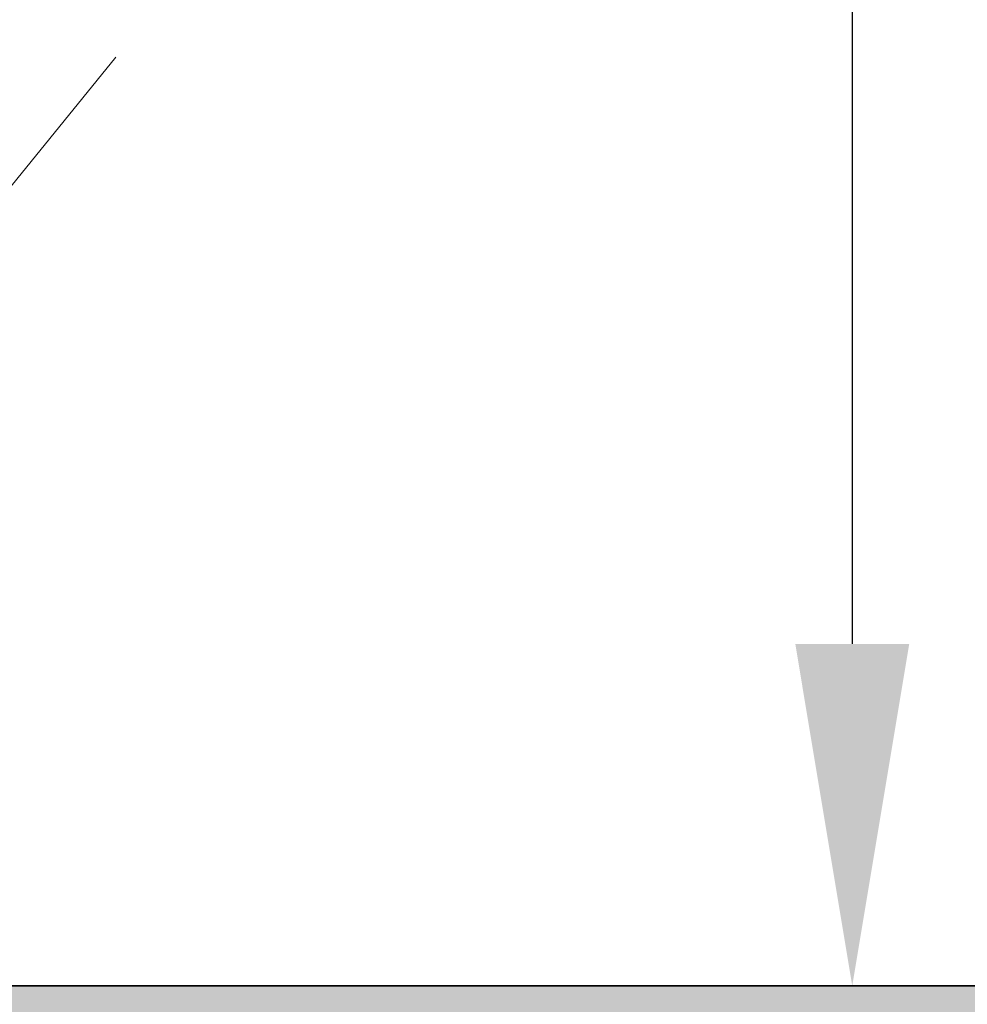
# Model space of a CAD drawing. Units: inches. Extents: x 2083 to 3317, y 1141 to 2115.
# Tile 79 of 256: x 2259 to 2292, y 1477 to 1512. Entities that reach past the tile are written whole.
import ezdxf

# ---------------------------------------------------------------- set-up
doc = ezdxf.new("R2010")
doc.units = ezdxf.units.IN
doc.linetypes.add('ACAD_ISO02W100', pattern=[15, 12, -3])
for name, color, linetype, lineweight in [('A-ANNO-DIMS', 2, 'Continuous', 18), ('A-FLOR-OPEN', 8, 'ACAD_ISO02W100', 13), ('A-WALL', 7, 'Continuous', 35)]:
    doc.layers.add(name, color=color, linetype=linetype, lineweight=lineweight)
doc.layers.add('A-WALL-PATT', color=251, linetype='Continuous', lineweight=13, true_color=0x636466)
doc.styles.get("Standard").update_dxf_attribs({"font": 'arial.ttf'})
doc.dimstyles.new('ISO-25', dxfattribs={"dimtxt": 12, "dimasz": 12, "dimexe": 1.25, "dimexo": 0.625, "dimtad": 1, "dimlunit": 3, "dimtxsty": 'Standard', "dimcen": 2.5, "dimadec": 0, "dimazin": 0, "dimtfac": 1, "dimtmove": 0, "dimatfit": 3, "dimfxl": 1, "dimarcsym": 0})

# ---------------------------------------------------------------- blocks, each defined once
blk = doc.blocks.new('*D30')
at = {"layer": 'A-ANNO-DIMS', "color": 0, "lineweight": -2, "transparency": 16777216}
for p, q in [((2240.018, 1445.274), (2240.018, 1448.046)), ((2254.329, 1445.274), (2254.329, 1448.046)), ((2228.018, 1446.796), (2216.018, 1446.796)), ((2240.018, 1446.796), (2254.329, 1446.796)), ((2266.329, 1446.796), (2413.765, 1446.796))]:
    blk.add_line(p, q, dxfattribs=at)
at = {"layer": 'A-ANNO-DIMS', "color": 0, "transparency": 16777216}
for points in [[(2228.018, 1448.796), (2228.018, 1444.796), (2240.018, 1446.796)], [(2266.329, 1448.796), (2266.329, 1444.796), (2254.329, 1446.796)]]:
    blk.add_solid(points, dxfattribs=at)
at = {"layer": 'Defpoints', "color": 0, "transparency": 16777216}
for p in [(2254.329, 1446.796), (2240.018, 1444.649), (2254.329, 1444.649)]:
    blk.add_point(p, dxfattribs=at)
at = {"layer": 'A-ANNO-DIMS', "color": 0, "transparency": 16777216, "insert": (2346.047, 1453.625), "char_height": 12, "attachment_point": 5}
blk.add_mtext('WC 1\'-2 1/2" TYP.', dxfattribs=at)
blk = doc.blocks.new('*D45')
at = {"layer": 'A-ANNO-DIMS', "color": 0, "lineweight": -2, "transparency": 16777216}
for p, q in [((2235.96, 1478.386), (2235.96, 1531.361)), ((2418.96, 1478.386), (2418.96, 1531.361)), ((2247.96, 1530.111), (2406.96, 1530.111))]:
    blk.add_line(p, q, dxfattribs=at)
at = {"layer": 'A-ANNO-DIMS', "color": 0, "transparency": 16777216}
for points in [[(2247.96, 1532.111), (2247.96, 1528.111), (2235.96, 1530.111)], [(2406.96, 1532.111), (2406.96, 1528.111), (2418.96, 1530.111)]]:
    blk.add_solid(points, dxfattribs=at)
at = {"layer": 'Defpoints', "color": 0, "transparency": 16777216}
for p in [(2418.96, 1530.111), (2235.96, 1477.761), (2418.96, 1477.761)]:
    blk.add_point(p, dxfattribs=at)
at = {"layer": 'A-ANNO-DIMS', "color": 0, "transparency": 16777216, "insert": (2327.46, 1536.867), "char_height": 12, "attachment_point": 5}
blk.add_mtext('15\'-3"', dxfattribs=at)
blk = doc.blocks.new('*D62')
at = {"layer": 'A-ANNO-DIMS', "color": 0, "lineweight": -2, "transparency": 16777216}
for p, q in [((2235.96, 1469.386), (2235.96, 1522.361)), ((2379.96, 1469.386), (2379.96, 1522.361)), ((2247.96, 1521.111), (2367.96, 1521.111))]:
    blk.add_line(p, q, dxfattribs=at)
at = {"layer": 'A-ANNO-DIMS', "color": 0, "transparency": 16777216}
for points in [[(2247.96, 1523.111), (2247.96, 1519.111), (2235.96, 1521.111)], [(2367.96, 1523.111), (2367.96, 1519.111), (2379.96, 1521.111)]]:
    blk.add_solid(points, dxfattribs=at)
at = {"layer": 'Defpoints', "color": 0, "transparency": 16777216}
for p in [(2379.96, 1521.111), (2235.96, 1468.761), (2379.96, 1468.761)]:
    blk.add_point(p, dxfattribs=at)
at = {"layer": 'A-ANNO-DIMS', "color": 0, "transparency": 16777216, "insert": (2307.96, 1527.863), "char_height": 12, "attachment_point": 5}
blk.add_mtext('12\'-0"', dxfattribs=at)
blk = doc.blocks.new('*D64')
at = {"layer": 'A-ANNO-DIMS', "color": 0, "lineweight": -2, "transparency": 16777216}
for p, q in [((2236.585, 1702.761), (2289.56, 1702.761)), ((2288.31, 1690.761), (2288.31, 1489.761)), ((2236.585, 1477.761), (2289.56, 1477.761))]:
    blk.add_line(p, q, dxfattribs=at)
at = {"layer": 'A-ANNO-DIMS', "color": 0, "transparency": 16777216}
for points in [[(2286.31, 1690.761), (2290.31, 1690.761), (2288.31, 1702.761)], [(2286.31, 1489.761), (2290.31, 1489.761), (2288.31, 1477.761)]]:
    blk.add_solid(points, dxfattribs=at)
at = {"layer": 'Defpoints', "color": 0, "transparency": 16777216}
for p in [(2235.96, 1702.761), (2235.96, 1477.761), (2288.31, 1477.761)]:
    blk.add_point(p, dxfattribs=at)
at = {"layer": 'A-ANNO-DIMS', "color": 0, "transparency": 16777216, "insert": (2281.558, 1590.261), "char_height": 12, "attachment_point": 5, "rotation": 90}
blk.add_mtext('18\'-9"', dxfattribs=at)

msp = doc.modelspace()

# ---------------------------------------------------------------- hatches: boundary and pattern name
at = {"layer": 'A-WALL-PATT'}
h = msp.add_hatch(color=256, dxfattribs=at)
h.dxf.hatch_style = 1
h.paths.add_polyline_path([(3126.96, 2020.761), (2748.96, 2020.761), (2604.96, 2020.761), (2226.96, 2020.761), (2226.96, 1702.761), (2466.96, 1702.761), (2466.96, 1582.761), (2418.96, 1582.761), (2418.96, 1477.761), (2226.96, 1477.761), (2226.96, 1263.261), (2544.96, 1263.261), (2544.96, 1411.761), (2604.96, 1411.761), (2685.96, 1411.761), (2685.96, 1420.761), (2604.96, 1420.761), (2604.96, 1573.761), (2604.96, 1702.761), (2604.96, 2011.761), (2748.96, 2011.761), (2748.96, 1702.761), (2862.96, 1702.761), (2862.96, 1621.761), (2871.96, 1621.761), (2871.96, 1702.761), (2883.96, 1702.761), (2883.96, 1706.939, -0.026459), (2883.96, 1711.761), (2757.96, 1711.761), (2757.96, 1807.761), (2787.96, 1807.761), (2787.96, 1812.261), (2757.96, 1812.261), (2757.96, 2011.761), (2877.96, 2011.761), (2877.96, 1812.261), (2847.96, 1812.261), (2847.96, 1807.761), (2889.836, 1807.761), (2889.836, 1812.261), (2882.46, 1812.261), (2882.46, 2011.761), (3117.96, 2011.761), (3117.96, 1812.261), (2937.836, 1812.261), (2937.836, 1807.761), (2995.71, 1807.761), (2995.71, 1796.118), (3000.21, 1796.118), (3000.21, 1807.761), (3117.96, 1807.761), (3117.96, 1711.761), (3000.21, 1711.761), (3000.21, 1760.118), (2998.573, 1760.118, -0.020711), (2995.71, 1760.118), (2995.71, 1711.761), (2931.96, 1711.761), (2931.96, 1702.761), (3126.96, 1702.761)])
h.paths.add_polyline_path([(2471.46, 2011.761), (2471.46, 1810.011), (2462.717, 1810.011), (2462.717, 1805.511), (2505.96, 1805.511), (2505.96, 1810.011), (2475.96, 1810.011), (2475.96, 2011.761), (2595.96, 2011.761), (2595.96, 1810.011), (2565.96, 1810.011), (2565.96, 1805.511), (2595.96, 1805.511), (2595.96, 1711.761), (2235.96, 1711.761), (2235.96, 1805.511), (2353.71, 1805.511), (2353.71, 1796.054), (2358.21, 1796.054), (2358.21, 1805.511), (2414.717, 1805.511), (2414.717, 1810.011), (2235.96, 1810.011), (2235.96, 2011.761)], flags=16)
h.paths.add_polyline_path([(2270.205, 1994.61), (2270.205, 1970.61), (2246.205, 1970.61), (2246.205, 1994.61)], flags=0)
edge = h.paths.add_edge_path(flags=0)
edge.add_ellipse((2332.027, 1899.798), major_axis=(-3.043, 3.043), ratio=0.168252, start_angle=-161.3322, end_angle=-156.3071, ccw=False)
edge.add_ellipse((2333.082, 1898.744), major_axis=(-1.055, 1.055), ratio=0.453532, start_angle=-123.371, end_angle=-94.1591)
edge = h.paths.add_edge_path(flags=0)
edge.add_ellipse((2332.027, 1968.876), major_axis=(3.043, 3.043), ratio=0.168252, start_angle=18.6678, end_angle=23.6929)
edge.add_spline(control_points=[(2332.926, 1970.691), (2332.227, 1970.336), (2330.894, 1969.659), (2328.413, 1970.932), (2327.204, 1967.749), (2324.71, 1969.956), (2322.533, 1967.012), (2320.013, 1971.296), (2317.68, 1968.158), (2316.041, 1967.102), (2315.427, 1966.81)], knot_values=[0, 0, 0, 0, 2.267059, 4.324559, 6.685584, 8.878641, 11.121502, 14.300359, 17.755284, 19.732645, 19.732645, 19.732645, 19.732645], degree=3, periodic=0)
edge.add_ellipse((2332.027, 1968.876), major_axis=(3.043, 3.043), ratio=0.168252, start_angle=18.6678, end_angle=23.6929, ccw=False)
edge.add_ellipse((2333.082, 1969.931), major_axis=(1.055, 1.055), ratio=0.453532, start_angle=56.629, end_angle=85.8409, ccw=False)
edge = h.paths.add_edge_path(flags=0)
edge.add_spline(control_points=[(2296.428, 1967.988), (2293.628, 1965.336), (2287.704, 1959.727), (2299.744, 1949.996), (2294.533, 1935.669), (2290.573, 1920.604), (2293.394, 1909.974), (2296.185, 1904.967)], knot_values=[0.099185, 0.099185, 0.099185, 0.099185, 0.345301, 0.619822, 0.982653, 1.386093, 1.810555, 1.810555, 1.810555, 1.810555], degree=3, periodic=0)
edge.add_spline(control_points=[(2296.185, 1904.967), (2297.384, 1902.619), (2298.001, 1901.949), (2298.553, 1901.468)], knot_values=[0.006246, 0.006246, 0.006246, 0.006246, 0.055476, 0.055476, 0.055476, 0.055476], degree=3, periodic=0)
edge.add_spline(control_points=[(2298.553, 1901.468), (2297.259, 1900.923), (2295.225, 1900.232), (2293.06, 1900.614), (2292.101, 1900.788), (2292.09, 1900.791)], knot_values=[0.312835, 0.312835, 0.312835, 0.312835, 0.40178, 0.474987, 0.475903, 0.475903, 0.475903, 0.475903], degree=3, periodic=0)
edge.add_arc((2292.794, 1904.664), 3.937, 215.4209, 259.6982, ccw=False)
edge.add_spline(control_points=[(2289.585, 1902.382), (2289.477, 1902.535), (2289.368, 1902.688), (2289.261, 1902.841)], knot_values=[0.102872, 0.102872, 0.102872, 0.102872, 0.116896, 0.116896, 0.116896, 0.116896], degree=3, periodic=0)
edge.add_spline(control_points=[(2289.261, 1902.841), (2288.687, 1902.55), (2287.64, 1902.02), (2285.881, 1901.874), (2283.853, 1901.504), (2281.72, 1899.711), (2278.467, 1899.493), (2276.157, 1901.883), (2272.259, 1899.804), (2267.778, 1901.843), (2262.244, 1900.184), (2257.415, 1901.782), (2254.318, 1900.726), (2253.178, 1900.337)], knot_values=[0, 0, 0, 0, 1.907977, 3.477176, 5.261074, 7.972851, 11.680248, 13.717921, 16.939592, 22.789562, 27.502503, 33.595215, 37.145618, 37.145618, 37.145618, 37.145618], degree=3, periodic=0)
edge.add_line((2253.178, 1900.337), (2250.244, 1902.841))
edge.add_line((2250.244, 1902.841), (2250.244, 1965.833))
edge.add_line((2250.244, 1965.833), (2253.178, 1968.337))
edge.add_spline(control_points=[(2253.178, 1968.337), (2254.318, 1967.948), (2257.415, 1966.892), (2262.244, 1968.49), (2267.778, 1966.831), (2271.527, 1968.537), (2273.876, 1967.828), (2274.207, 1967.728)], knot_values=[0, 0, 0, 0, 0.09018, 0.244935, 0.364644, 0.513233, 0.537855, 0.537855, 0.537855, 0.537855], degree=3, periodic=0)
edge.add_arc((2274.353, 1963.793), 3.937, 72.0511, 92.1279, ccw=False)
edge.add_arc((2281.297, 1985.23), 18.596, 252.0511, 288.5657)
edge.add_arc((2292.317, 1956.029), 12.646, 71.0268, 113.7782, ccw=False)
edge = h.paths.add_edge_path(flags=0)
edge.add_spline(control_points=[(2274.899, 1951.856), (2275.066, 1951.617), (2275.233, 1951.377), (2275.398, 1951.136)], knot_values=[1.409916, 1.409916, 1.409916, 1.409916, 1.43159, 1.43159, 1.43159, 1.43159], degree=3, periodic=0)
edge.add_spline(control_points=[(2275.398, 1951.136), (2275.792, 1950.562), (2276.179, 1949.984), (2276.546, 1949.397)], knot_values=[1.358238, 1.358238, 1.358238, 1.358238, 1.409916, 1.409916, 1.409916, 1.409916], degree=3, periodic=0)
edge.add_line((2276.546, 1949.397), (2277.437, 1947.862))
edge.add_spline(control_points=[(2277.437, 1947.862), (2276.304, 1945.673), (2274.64, 1942.427), (2274.632, 1938.094), (2272.799, 1930.852), (2274.356, 1943.897), (2275.948, 1947.923), (2276.546, 1949.397)], knot_values=[0.005632, 0.005632, 0.005632, 0.005632, 0.186014, 0.266002, 0.357087, 0.59639, 0.739732, 0.739732, 0.739732, 0.739732], degree=3, periodic=0)
edge.add_spline(control_points=[(2276.546, 1949.397), (2276.179, 1949.984), (2275.792, 1950.562), (2275.398, 1951.136)], knot_values=[1.358238, 1.358238, 1.358238, 1.358238, 1.409916, 1.409916, 1.409916, 1.409916], degree=3, periodic=0)
edge.add_spline(control_points=[(2275.398, 1951.136), (2274.943, 1950.08), (2274.208, 1948.025), (2273.935, 1944.851), (2272.469, 1937.627), (2273.466, 1945.696), (2274.701, 1951.059), (2274.899, 1951.856)], knot_values=[0.104364, 0.104364, 0.104364, 0.104364, 0.189636, 0.269624, 0.36071, 0.600013, 0.644622, 0.644622, 0.644622, 0.644622], degree=3, periodic=0)
h.paths.add_polyline_path([(2269.168, 1963.128, -0.357527), (2268.171, 1960.976, -0.092561), (2268.171, 1939.436, -0.357527), (2269.168, 1937.285, -0.357527), (2267.016, 1938.282, -0.164785), (2254.686, 1938.282, -0.357527), (2252.534, 1937.285, -0.357527), (2253.531, 1939.436, -0.092561), (2253.531, 1960.976, -0.357527), (2252.534, 1963.128, -0.357527), (2254.686, 1962.131, -0.164785), (2267.016, 1962.131, -0.357527)], flags=0)
h.paths.add_polyline_path([(2248.874, 1967.802), (2248.874, 1957.028), (2249.458, 1957.028), (2249.458, 1911.647), (2248.874, 1911.647), (2248.874, 1900.873), (2246.512, 1900.873, 0.197327), (2244.15, 1902.457), (2244.15, 1966.218, 0.197327), (2246.512, 1967.802)], flags=0)
h.paths.add_polyline_path([(2269.168, 1931.389, -0.357527), (2268.171, 1929.238, -0.092561), (2268.171, 1907.698, -0.357527), (2269.168, 1905.547, -0.357527), (2267.016, 1906.544, -0.164785), (2254.686, 1906.544, -0.357527), (2252.534, 1905.547, -0.357527), (2253.531, 1907.698, -0.092561), (2253.531, 1929.238, -0.357527), (2252.534, 1931.389, -0.357527), (2254.686, 1930.392, -0.164785), (2267.016, 1930.392, -0.357527)], flags=0)
edge = h.paths.add_edge_path(flags=0)
edge.add_spline(control_points=[(2276.197, 1906.724), (2276.168, 1909.029), (2276.114, 1913.372), (2270.598, 1924.925), (2273.905, 1919.013), (2275.922, 1916.262), (2275.475, 1912.402), (2277.258, 1910.381), (2276.696, 1908.225), (2276.646, 1906.813), (2276.618, 1906.008)], knot_values=[0, 0, 0, 0, 8.61026, 16.221274, 18.843057, 23.804898, 27.440828, 29.356102, 31.203478, 33.650687, 33.650687, 33.650687, 33.650687], degree=3, periodic=0)
edge.add_spline(control_points=[(2276.618, 1906.008), (2276.623, 1905.624), (2276.498, 1904.629), (2275.442, 1903.855), (2274.937, 1903.08), (2274.859, 1902.841)], knot_values=[0.156488, 0.156488, 0.156488, 0.156488, 0.184398, 0.231376, 0.250598, 0.250598, 0.250598, 0.250598], degree=3, periodic=0)
edge.add_line((2274.859, 1902.841), (2276.506, 1902.841))
edge.add_spline(control_points=[(2276.506, 1902.841), (2276.788, 1903.085), (2277.665, 1904.125), (2278.25, 1904.341), (2277.654, 1908.527), (2278.156, 1906.228), (2278.1, 1905.286), (2278.847, 1904.069), (2277.857, 1903.415), (2277.874, 1902.991), (2277.904, 1902.841)], knot_values=[0.059574, 0.059574, 0.059574, 0.059574, 0.080753, 0.103741, 0.16972, 0.176036, 0.207137, 0.240474, 0.262341, 0.27366, 0.27366, 0.27366, 0.27366], degree=3, periodic=0)
edge.add_line((2277.904, 1902.841), (2280.03, 1902.841))
edge.add_spline(control_points=[(2280.03, 1902.841), (2279.888, 1903.088), (2279.499, 1903.982), (2280.152, 1905.939), (2278.104, 1909.658), (2279.762, 1907.185), (2280.328, 1904.875), (2280.485, 1903.49), (2281.463, 1903.249), (2281.758, 1902.936), (2281.834, 1902.841)], knot_values=[0.013856, 0.013856, 0.013856, 0.013856, 0.034874, 0.088867, 0.107879, 0.126738, 0.158714, 0.193757, 0.217487, 0.226722, 0.226722, 0.226722, 0.226722], degree=3, periodic=0)
edge.add_spline(control_points=[(2281.834, 1902.841), (2281.788, 1902.827), (2281.647, 1902.783), (2281.396, 1902.859), (2281.088, 1902.985), (2280.721, 1903.061), (2280.333, 1903.026), (2280.125, 1902.899), (2280.03, 1902.841)], knot_values=[0, 0, 0, 0, 0.14413, 0.435517, 0.749276, 1.153046, 1.548371, 1.878348, 1.878348, 1.878348, 1.878348], degree=3, periodic=0)
edge.add_line((2280.03, 1902.841), (2277.904, 1902.841))
edge.add_spline(control_points=[(2277.904, 1902.841), (2277.893, 1902.796), (2277.865, 1902.68), (2277.607, 1902.687), (2277.274, 1902.801), (2276.838, 1902.62), (2276.584, 1902.789), (2276.506, 1902.841)], knot_values=[0, 0, 0, 0, 0.127189, 0.326199, 0.628009, 1.24357, 1.515331, 1.515331, 1.515331, 1.515331], degree=3, periodic=0)
edge.add_line((2276.506, 1902.841), (2274.859, 1902.841))
edge.add_spline(control_points=[(2274.859, 1902.841), (2274.814, 1902.899), (2274.725, 1903.013), (2274.493, 1903.119), (2274.244, 1902.961), (2273.937, 1903.185), (2273.614, 1902.983), (2273.408, 1902.883), (2273.322, 1902.841)], knot_values=[0, 0, 0, 0, 0.21843, 0.436957, 0.687977, 0.990379, 1.398396, 1.69185, 1.69185, 1.69185, 1.69185], degree=3, periodic=0)
edge.add_spline(control_points=[(2273.322, 1902.841), (2273.617, 1903.446), (2274.274, 1904.538), (2276.027, 1904.574), (2276.207, 1906.584), (2276.197, 1906.724)], knot_values=[0.012227, 0.012227, 0.012227, 0.012227, 0.059472, 0.106218, 0.134458, 0.134458, 0.134458, 0.134458], degree=3, periodic=0)
h.paths.add_polyline_path([(2270.776, 1897.79), (2270.776, 1873.79), (2246.776, 1873.79), (2246.776, 1897.79)], flags=0)
h.paths.add_polyline_path([(2353.71, 1760.005), (2353.71, 1760.054), (2358.21, 1760.054, -0.033729)], flags=0)
h.paths.add_polyline_path([(2321.819, 1737.529), (2341.995, 1737.529, -0.414214), (2343.203, 1736.321), (2343.203, 1721.021, -0.414214), (2341.995, 1719.813), (2321.819, 1719.813, -0.414214), (2320.611, 1721.021), (2320.611, 1736.321, -0.414214)], flags=0)
h.paths.add_polyline_path([(2324.235, 1736.321), (2339.579, 1736.321, -0.414214), (2341.995, 1733.905), (2341.995, 1725.45, -0.414214), (2339.579, 1723.034), (2333.681, 1723.034), (2333.845, 1722.045, -0.870646), (2335.425, 1721.826, -0.767327), (2333.923, 1721.423), (2331.291, 1721.423, -0.767327), (2329.788, 1721.826, -0.870646), (2331.368, 1722.045), (2331.533, 1723.034), (2324.235, 1723.034, -0.414214), (2321.819, 1725.45), (2321.819, 1733.905, -0.414214)], flags=0)
h.paths.add_polyline_path([(2570.484, 1928.615), (2589.684, 1928.615), (2590.169, 1928.615), (2590.169, 1904.993), (2570.484, 1904.993)], flags=0)
h.paths.add_polyline_path([(2574.447, 1927.264, -1), (2572.829, 1927.264, -1)], flags=0)
h.paths.add_polyline_path([(2573.09, 1926.941), (2573.925, 1927.776), (2574.148, 1927.553), (2573.313, 1926.718)], flags=0)
h.paths.add_polyline_path([(2578.779, 1919.73, -1), (2571.592, 1919.73, -1)], flags=0)
h.paths.add_polyline_path([(2578.385, 1919.73, -1), (2571.985, 1919.73, -1)], flags=0)
h.paths.add_polyline_path([(2331.596, 1729.476, -1), (2333.618, 1729.476, -1)], flags=0)
h.paths.add_polyline_path([(2578.034, 1927.264, -1), (2576.416, 1927.264, -1)], flags=0)
h.paths.add_polyline_path([(2576.689, 1927.531), (2576.912, 1927.754), (2577.747, 1926.919), (2577.524, 1926.696)], flags=0)
h.paths.add_polyline_path([(2578.139, 1909.86, -1), (2572.232, 1909.86, -1)], flags=0)
h.paths.add_polyline_path([(2577.745, 1909.86, -1), (2572.625, 1909.86, -1)], flags=0)
h.paths.add_polyline_path([(2583.798, 1927.264, -1), (2582.179, 1927.264, -1)], flags=0)
h.paths.add_polyline_path([(2582.719, 1927.754), (2583.554, 1926.919), (2583.331, 1926.696), (2582.496, 1927.531)], flags=0)
h.paths.add_polyline_path([(2582.496, 1927.531), (2582.719, 1927.754), (2583.554, 1926.919), (2583.331, 1926.696)], flags=0)
h.paths.add_polyline_path([(2587.739, 1920.53, -1), (2581.832, 1920.53, -1)], flags=0)
h.paths.add_polyline_path([(2587.345, 1920.53, -1), (2582.225, 1920.53, -1)], flags=0)
h.paths.add_polyline_path([(2587.385, 1927.264, -1), (2585.766, 1927.264, -1)], flags=0)
h.paths.add_polyline_path([(2586.082, 1926.98), (2586.917, 1927.815), (2587.14, 1927.593), (2586.305, 1926.758)], flags=0)
h.paths.add_polyline_path([(2588.379, 1910.66, -1), (2581.192, 1910.66, -1)], flags=0)
h.paths.add_polyline_path([(2587.985, 1910.66, -1), (2581.585, 1910.66, -1)], flags=0)
h.paths.add_polyline_path([(2417.168, 1729.478), (2437.344, 1729.478, -0.414214), (2438.552, 1728.27), (2438.552, 1712.969, -0.414214), (2437.344, 1711.761), (2417.168, 1711.761, -0.414214), (2415.96, 1712.969), (2415.96, 1728.27, -0.414214)], flags=0)
h.paths.add_polyline_path([(2419.584, 1728.27), (2434.928, 1728.27, -0.414214), (2437.344, 1725.854), (2437.344, 1717.398, -0.414214), (2434.928, 1714.983), (2429.029, 1714.983), (2429.194, 1713.994, -0.870646), (2430.774, 1713.775, -0.767327), (2429.271, 1713.372), (2426.64, 1713.372, -0.767327), (2425.137, 1713.775, -0.870646), (2426.717, 1713.994), (2426.882, 1714.983), (2419.584, 1714.983, -0.414214), (2417.168, 1717.398), (2417.168, 1725.854, -0.414214)], flags=0)
h.paths.add_polyline_path([(2419.584, 1728.27), (2434.928, 1728.27, -0.414214), (2437.344, 1725.854), (2437.344, 1717.398, -0.414214), (2434.928, 1714.983), (2429.029, 1714.983), (2428.358, 1719.009), (2427.553, 1719.009), (2426.882, 1714.983), (2419.584, 1714.983, -0.414214), (2417.168, 1717.398), (2417.168, 1725.854, -0.414214)], flags=0)
h.paths.add_polyline_path([(2426.944, 1721.425, -1), (2428.967, 1721.425, -1)], flags=0)
h.paths.add_polyline_path([(2475.96, 1702.761), (2595.96, 1702.761), (2595.96, 1582.761), (2475.96, 1582.761)], flags=16)
h.paths.add_polyline_path([(2427.96, 1573.761), (2595.96, 1573.761), (2595.96, 1468.761), (2595.96, 1420.761), (2384.46, 1420.761), (2384.46, 1468.761), (2427.96, 1468.761)], flags=16)
h.paths.add_polyline_path([(2379.96, 1468.761), (2379.96, 1420.761), (2235.96, 1420.761), (2235.96, 1468.761)], flags=16)
h.paths.add_polyline_path([(2317.816, 1466.696), (2337.992, 1466.696, -0.414214), (2339.2, 1465.488), (2339.2, 1450.187, -0.414214), (2337.992, 1448.979), (2317.816, 1448.979, -0.414214), (2316.608, 1450.187), (2316.608, 1465.488, -0.414214)], flags=0)
h.paths.add_polyline_path([(2320.232, 1465.488), (2335.576, 1465.488, -0.414214), (2337.992, 1463.072), (2337.992, 1454.616, -0.414214), (2335.576, 1452.2), (2329.677, 1452.2), (2329.842, 1451.212, -0.870646), (2331.422, 1450.992, -0.767327), (2329.92, 1450.59), (2327.288, 1450.59, -0.767327), (2325.785, 1450.992, -0.870646), (2327.365, 1451.212), (2327.53, 1452.2), (2320.232, 1452.2, -0.414214), (2317.816, 1454.616), (2317.816, 1463.072, -0.414214)], flags=0)
h.paths.add_polyline_path([(2320.232, 1465.488), (2335.576, 1465.488, -0.414214), (2337.992, 1463.072), (2337.992, 1454.616, -0.414214), (2335.576, 1452.2), (2329.677, 1452.2), (2329.006, 1456.227), (2328.201, 1456.227), (2327.53, 1452.2), (2320.232, 1452.2, -0.414214), (2317.816, 1454.616), (2317.816, 1463.072, -0.414214)], flags=0)
h.paths.add_polyline_path([(2327.593, 1458.643, -1), (2329.615, 1458.643, -1)], flags=0)
h.paths.add_polyline_path([(2244.412, 1433.34), (2241.921, 1433.34, -0.414214), (2240.018, 1435.244), (2240.018, 1440.953, -0.414211), (2241.921, 1442.856), (2244.412, 1442.856, -1.976472)], flags=0)
h.paths.add_polyline_path([(2245.357, 1434.398, -0.414214), (2245.357, 1441.799, -2.144098)], flags=0)
h.paths.add_polyline_path([(2535.96, 1416.261), (2535.96, 1272.261), (2235.96, 1272.261), (2235.96, 1416.261)], flags=16)
h.paths.add_polyline_path([(2260.12, 1384.293), (2260.12, 1362.039), (2237.865, 1362.039), (2237.865, 1384.293)], flags=0)
edge = h.paths.add_edge_path(flags=0)
edge.add_line((2318.252, 1362.093), (2318.146, 1362.001))
edge.add_ellipse((2317.445, 1360.431), major_axis=(2.822, 2.822), ratio=0.168252, start_angle=18.6678, end_angle=20.9481, ccw=False)
edge.add_ellipse((2318.423, 1361.409), major_axis=(0.978, 0.978), ratio=0.453532, start_angle=56.629, end_angle=70.2262, ccw=False)
edge = h.paths.add_edge_path(flags=0)
edge.add_line((2319.107, 1295.571), (2319.015, 1295.677))
edge.add_ellipse((2317.445, 1296.378), major_axis=(-2.822, 2.822), ratio=0.168252, start_angle=-161.3322, end_angle=-159.0519, ccw=False)
edge.add_ellipse((2318.423, 1295.4), major_axis=(-0.978, 0.978), ratio=0.453532, start_angle=-123.371, end_angle=-109.7738)
edge = h.paths.add_edge_path(flags=0)
edge.add_spline(control_points=[(2284.21, 1301.17), (2284.581, 1300.445), (2284.891, 1299.892), (2285.16, 1299.461)], knot_values=[0.039066, 0.039066, 0.039066, 0.039066, 0.055476, 0.055476, 0.055476, 0.055476], degree=3, periodic=0)
edge.add_line((2285.16, 1299.461), (2284.21, 1301.17))
edge = h.paths.add_edge_path(flags=0)
edge.add_line((2280.412, 1297.298), (2283.37, 1297.036))
edge.add_line((2283.37, 1297.036), (2286.406, 1297.926))
edge.add_spline(control_points=[(2286.406, 1297.926), (2285.305, 1297.463), (2284.345, 1297.129), (2283.37, 1297.036)], knot_values=[0.394369, 0.394369, 0.394369, 0.394369, 0.475903, 0.475903, 0.475903, 0.475903], degree=3, periodic=0)
edge.add_spline(control_points=[(2283.37, 1297.036), (2283.281, 1297.028), (2282.316, 1296.957), (2281.313, 1297.134), (2280.423, 1297.296), (2280.412, 1297.298)], knot_values=[0.312835, 0.312835, 0.312835, 0.312835, 0.320246, 0.393453, 0.394369, 0.394369, 0.394369, 0.394369], degree=3, periodic=0)
edge = h.paths.add_edge_path(flags=0)
edge.add_line((2284.436, 1359.607), (2280.446, 1355.328))
edge.add_line((2280.446, 1355.328), (2279.58, 1351.018))
edge.add_line((2279.58, 1351.018), (2282.413, 1346.58))
edge.add_spline(control_points=[(2282.413, 1346.58), (2283.153, 1345.589), (2284.253, 1344.029), (2284.801, 1342.387), (2284.935, 1341.806)], knot_values=[1.240098, 1.240098, 1.240098, 1.240098, 1.332892, 1.382712, 1.382712, 1.382712, 1.382712], degree=3, periodic=0)
edge.add_spline(control_points=[(2284.935, 1341.806), (2285.319, 1340.141), (2285.233, 1338.409), (2284.91, 1336.654)], knot_values=[1.097484, 1.097484, 1.097484, 1.097484, 1.240098, 1.240098, 1.240098, 1.240098], degree=3, periodic=0)
edge.add_spline(control_points=[(2284.91, 1336.654), (2284.587, 1334.899), (2284.027, 1333.12), (2283.463, 1331.361)], knot_values=[0.95487, 0.95487, 0.95487, 0.95487, 1.097484, 1.097484, 1.097484, 1.097484], degree=3, periodic=0)
edge.add_line((2283.463, 1331.361), (2281.89, 1326.153))
edge.add_line((2281.89, 1326.153), (2280.756, 1321.056))
edge.add_line((2280.756, 1321.056), (2280.299, 1316.002))
edge.add_line((2280.299, 1316.002), (2280.716, 1310.95))
edge.add_line((2280.716, 1310.95), (2282.028, 1305.972))
edge.add_line((2282.028, 1305.972), (2284.21, 1301.17))
edge.add_spline(control_points=[(2284.21, 1301.17), (2283.341, 1302.73), (2282.612, 1304.336), (2282.028, 1305.972)], knot_values=[0.099185, 0.099185, 0.099185, 0.099185, 0.241799, 0.241799, 0.241799, 0.241799], degree=3, periodic=0)
edge.add_spline(control_points=[(2282.028, 1305.972), (2281.444, 1307.608), (2281.005, 1309.273), (2280.716, 1310.95)], knot_values=[0.241799, 0.241799, 0.241799, 0.241799, 0.384413, 0.384413, 0.384413, 0.384413], degree=3, periodic=0)
edge.add_spline(control_points=[(2280.716, 1310.95), (2280.433, 1312.588), (2280.289, 1314.277), (2280.299, 1315.962), (2280.299, 1316.002)], knot_values=[0.384413, 0.384413, 0.384413, 0.384413, 0.523647, 0.527028, 0.527028, 0.527028, 0.527028], degree=3, periodic=0)
edge.add_spline(control_points=[(2280.299, 1316.002), (2280.312, 1317.687), (2280.478, 1319.368), (2280.756, 1321.056)], knot_values=[0.527028, 0.527028, 0.527028, 0.527028, 0.669642, 0.669642, 0.669642, 0.669642], degree=3, periodic=0)
edge.add_spline(control_points=[(2280.756, 1321.056), (2281.035, 1322.744), (2281.426, 1324.44), (2281.89, 1326.153)], knot_values=[0.669642, 0.669642, 0.669642, 0.669642, 0.812256, 0.812256, 0.812256, 0.812256], degree=3, periodic=0)
edge.add_spline(control_points=[(2281.89, 1326.153), (2282.264, 1327.533), (2282.788, 1329.262), (2283.353, 1331.018), (2283.463, 1331.361)], knot_values=[0.812256, 0.812256, 0.812256, 0.812256, 0.927087, 0.95487, 0.95487, 0.95487, 0.95487], degree=3, periodic=0)
edge.add_line((2283.463, 1331.361), (2284.91, 1336.654))
edge.add_line((2284.91, 1336.654), (2284.935, 1341.806))
edge.add_line((2284.935, 1341.806), (2282.413, 1346.58))
edge.add_spline(control_points=[(2282.413, 1346.58), (2281.275, 1348.104), (2280.078, 1349.57), (2279.58, 1351.018)], knot_values=[1.382712, 1.382712, 1.382712, 1.382712, 1.525326, 1.525326, 1.525326, 1.525326], degree=3, periodic=0)
edge.add_spline(control_points=[(2279.58, 1351.018), (2279.443, 1351.415), (2279.136, 1352.857), (2279.735, 1354.29), (2280.446, 1355.328)], knot_values=[1.525326, 1.525326, 1.525326, 1.525326, 1.564439, 1.667941, 1.667941, 1.667941, 1.667941], degree=3, periodic=0)
edge.add_spline(control_points=[(2280.446, 1355.328), (2281.426, 1356.758), (2282.931, 1358.183), (2284.436, 1359.607)], knot_values=[1.667941, 1.667941, 1.667941, 1.667941, 1.810555, 1.810555, 1.810555, 1.810555], degree=3, periodic=0)
edge.add_arc((2280.623, 1348.518), 11.726, 71.0268, 113.7782)
edge.add_arc((2270.405, 1375.595), 17.244, 252.0511, 288.5657, ccw=False)
edge.add_arc((2263.966, 1355.718), 3.651, 72.0511, 92.1279)
edge.add_arc((2263.966, 1355.718), 3.651, 92.1279, 177.9851)
edge.add_spline(control_points=[(2260.318, 1355.846), (2260.26, 1354.221), (2260.551, 1350.187), (2262.999, 1346.766), (2264.473, 1344.649)], knot_values=[1.43159, 1.43159, 1.43159, 1.43159, 1.564144, 1.770695, 1.770695, 1.770695, 1.770695], degree=3, periodic=0)
edge.add_line((2264.473, 1344.649), (2264.936, 1343.983))
edge.add_spline(control_points=[(2263.801, 1340.248), (2263.843, 1340.514), (2264.067, 1341.756), (2264.513, 1343.002), (2264.935, 1343.981)], knot_values=[0.53657, 0.53657, 0.53657, 0.53657, 0.559349, 0.644622, 0.644622, 0.644622, 0.644622], degree=3, periodic=0)
edge.add_spline(control_points=[(2264.935, 1343.981), (2265.118, 1343.715), (2265.299, 1343.448), (2265.477, 1343.179)], knot_values=[1.384077, 1.384077, 1.384077, 1.384077, 1.409916, 1.409916, 1.409916, 1.409916], degree=3, periodic=0)
edge.add_spline(control_points=[(2265.477, 1343.179), (2265.655, 1342.911), (2265.829, 1342.641), (2265.999, 1342.369)], knot_values=[1.358238, 1.358238, 1.358238, 1.358238, 1.384077, 1.384077, 1.384077, 1.384077], degree=3, periodic=0)
edge.add_line((2265.999, 1342.369), (2266.826, 1340.946))
edge.add_spline(control_points=[(2266.826, 1340.946), (2268.894, 1337.09), (2271.398, 1325.843), (2270.516, 1310.569), (2275.919, 1301.861), (2277.79, 1299.199)], knot_values=[0.116896, 0.116896, 0.116896, 0.116896, 0.472987, 1.050969, 1.313793, 1.313793, 1.313793, 1.313793], degree=3, periodic=0)
edge.add_spline(control_points=[(2277.79, 1299.199), (2277.839, 1299.128), (2277.889, 1299.057), (2277.94, 1298.987)], knot_values=[0.109884, 0.109884, 0.109884, 0.109884, 0.116896, 0.116896, 0.116896, 0.116896], degree=3, periodic=0)
edge.add_line((2277.94, 1298.987), (2277.789, 1299.199))
edge.add_spline(control_points=[(2277.789, 1299.199), (2277.257, 1298.929), (2276.286, 1298.438), (2275.039, 1298.334), (2274.383, 1298.239), (2274.215, 1298.209)], knot_values=[33.12187, 33.12187, 33.12187, 33.12187, 35.029056, 36.598255, 37.144827, 37.144827, 37.144827, 37.144827], degree=3, periodic=0)
edge.add_line((2274.215, 1298.209), (2273.073, 1297.893))
edge.add_spline(control_points=[(2273.073, 1297.893), (2272.323, 1297.58), (2271.039, 1296.511), (2269.248, 1296.226), (2268.423, 1296.375)], knot_values=[26.532584, 26.532584, 26.532584, 26.532584, 29.198919, 31.839101, 31.839101, 31.839101, 31.839101], degree=3, periodic=0)
edge.add_line((2268.423, 1296.375), (2263.879, 1297.458))
edge.add_spline(control_points=[(2263.879, 1297.458), (2263.556, 1297.359), (2261.86, 1296.839), (2260.239, 1297.282), (2258.933, 1297.516)], knot_values=[15.919551, 15.919551, 15.919551, 15.919551, 16.939592, 21.226067, 21.226067, 21.226067, 21.226067], degree=3, periodic=0)
edge.add_line((2258.933, 1297.516), (2254.055, 1297.329))
edge.add_spline(control_points=[(2254.055, 1297.329), (2253.756, 1297.296), (2252.114, 1297.165), (2250.462, 1297.544), (2249.13, 1297.668)], knot_values=[5.306517, 5.306517, 5.306517, 5.306517, 6.276435, 10.613034, 10.613034, 10.613034, 10.613034], degree=3, periodic=0)
edge.add_line((2249.13, 1297.668), (2244.332, 1296.878))
edge.add_line((2244.332, 1296.878), (2241.611, 1299.199))
edge.add_line((2241.611, 1299.199), (2241.611, 1357.609))
edge.add_line((2241.611, 1357.609), (2244.332, 1359.931))
edge.add_line((2244.332, 1359.931), (2252.729, 1359.543))
edge.add_spline(control_points=[(2252.729, 1359.543), (2252.871, 1359.546), (2253.306, 1359.548), (2253.74, 1359.514), (2254.032, 1359.482)], knot_values=[0.233291, 0.233291, 0.233291, 0.233291, 0.244935, 0.268927, 0.268927, 0.268927, 0.268927], degree=3, periodic=0)
edge.add_line((2254.032, 1359.482), (2259.587, 1359.416))
edge.add_spline(control_points=[(2259.587, 1359.416), (2260.677, 1359.629), (2262.073, 1359.897), (2263.524, 1359.459), (2263.83, 1359.366)], knot_values=[0.422516, 0.422516, 0.422516, 0.422516, 0.513233, 0.537855, 0.537855, 0.537855, 0.537855], degree=3, periodic=0)
edge.add_arc((2263.966, 1355.718), 3.651, 72.0511, 92.1279, ccw=False)
edge.add_arc((2270.405, 1375.595), 17.244, 252.0511, 288.5657)
edge.add_arc((2280.623, 1348.518), 11.726, 71.0268, 113.7782, ccw=False)
h.paths.add_polyline_path([(2240.341, 1359.435), (2240.341, 1349.444), (2240.882, 1349.444), (2240.882, 1307.365), (2240.341, 1307.365), (2240.341, 1297.374), (2238.15, 1297.374, 0.197327), (2235.96, 1298.843), (2235.96, 1357.966, 0.197327), (2238.15, 1359.435)], flags=0)
h.paths.add_polyline_path([(2259.158, 1355.101, -0.357527), (2258.233, 1353.106, -0.092561), (2258.233, 1333.133, -0.357527), (2259.158, 1331.138, -0.357527), (2257.163, 1332.062, -0.164785), (2245.729, 1332.062, -0.357527), (2243.735, 1331.138, -0.357527), (2244.659, 1333.133, -0.092561), (2244.659, 1353.106, -0.357527), (2243.735, 1355.101, -0.357527), (2245.729, 1354.176, -0.164785), (2257.163, 1354.176, -0.357527)], flags=0)
edge = h.paths.add_edge_path(flags=0)
edge.add_line((2265.999, 1342.369), (2266.826, 1340.946))
edge.add_line((2266.826, 1340.946), (2265.308, 1337.814))
edge.add_line((2265.308, 1337.814), (2264.358, 1334.653))
edge.add_line((2264.358, 1334.653), (2264.262, 1333.8))
edge.add_spline(control_points=[(2264.262, 1333.8), (2264.208, 1333.187), (2264.162, 1332.366), (2264.007, 1331.414), (2263.969, 1331.202)], knot_values=[0.464444, 0.464444, 0.464444, 0.464444, 0.516691, 0.531608, 0.531608, 0.531608, 0.531608], degree=3, periodic=0)
edge.add_spline(control_points=[(2263.969, 1331.202), (2263.775, 1330.119), (2263.424, 1328.791), (2263.257, 1328.531), (2263.234, 1328.515)], knot_values=[0.372682, 0.372682, 0.372682, 0.372682, 0.44885, 0.464444, 0.464444, 0.464444, 0.464444], degree=3, periodic=0)
edge.add_spline(control_points=[(2263.234, 1328.515), (2263.096, 1328.42), (2263.131, 1329.301), (2263.275, 1330.616)], knot_values=[0.280919, 0.280919, 0.280919, 0.280919, 0.372682, 0.372682, 0.372682, 0.372682], degree=3, periodic=0)
edge.add_spline(control_points=[(2263.275, 1330.616), (2263.419, 1331.93), (2263.672, 1333.677), (2263.97, 1335.315)], knot_values=[0.189157, 0.189157, 0.189157, 0.189157, 0.280919, 0.280919, 0.280919, 0.280919], degree=3, periodic=0)
edge.add_spline(control_points=[(2263.97, 1335.315), (2264.1, 1336.032), (2264.419, 1337.622), (2264.755, 1338.864), (2264.947, 1339.491)], knot_values=[0.097394, 0.097394, 0.097394, 0.097394, 0.137578, 0.189157, 0.189157, 0.189157, 0.189157], degree=3, periodic=0)
edge.add_spline(control_points=[(2264.947, 1339.491), (2265.29, 1340.606), (2265.644, 1341.494), (2265.999, 1342.369)], knot_values=[0.005632, 0.005632, 0.005632, 0.005632, 0.097394, 0.097394, 0.097394, 0.097394], degree=3, periodic=0)
h.paths.add_polyline_path([(2259.158, 1325.671, -0.357527), (2258.233, 1323.676, -0.092561), (2258.233, 1303.703, -0.357527), (2259.158, 1301.708, -0.357527), (2257.163, 1302.633, -0.164785), (2245.729, 1302.633, -0.357527), (2243.735, 1301.708, -0.357527), (2244.659, 1303.703, -0.092561), (2244.659, 1323.676, -0.357527), (2243.735, 1325.671, -0.357527), (2245.729, 1324.747, -0.164785), (2257.163, 1324.747, -0.357527)], flags=0)
edge = h.paths.add_edge_path(flags=0)
edge.add_spline(control_points=[(2261.709, 1317.311), (2261.679, 1317.418), (2261.762, 1317.389), (2262.491, 1316.09), (2262.962, 1315.301)], knot_values=[14.955861, 14.955861, 14.955861, 14.955861, 16.221274, 18.694826, 18.694826, 18.694826, 18.694826], degree=3, periodic=0)
edge.add_spline(control_points=[(2262.962, 1315.301), (2262.99, 1315.254), (2263.702, 1314.067), (2264.349, 1313.127), (2264.73, 1312.164)], knot_values=[18.694826, 18.694826, 18.694826, 18.694826, 18.843057, 22.433791, 22.433791, 22.433791, 22.433791], degree=3, periodic=0)
edge.add_spline(control_points=[(2264.73, 1312.164), (2264.876, 1311.796), (2265.177, 1310.77), (2265.143, 1309.559), (2265.248, 1308.824)], knot_values=[22.433791, 22.433791, 22.433791, 22.433791, 23.804898, 26.172756, 26.172756, 26.172756, 26.172756], degree=3, periodic=0)
edge.add_line((2265.248, 1308.824), (2265.851, 1307.172))
edge.add_spline(control_points=[(2265.851, 1307.172), (2266.065, 1306.822), (2266.384, 1306.332), (2266.424, 1305.781), (2266.42, 1305.611)], knot_values=[28.062562, 28.062562, 28.062562, 28.062562, 29.356102, 29.911721, 29.911721, 29.911721, 29.911721], degree=3, periodic=0)
edge.add_spline(control_points=[(2266.42, 1305.611), (2266.416, 1305.433), (2266.394, 1305.25), (2266.365, 1305.066)], knot_values=[29.911721, 29.911721, 29.911721, 29.911721, 30.497837, 30.497837, 30.497837, 30.497837], degree=3, periodic=0)
edge.add_line((2266.365, 1305.066), (2266.066, 1302.136))
edge.add_spline(control_points=[(2266.066, 1302.136), (2266.071, 1301.78), (2265.998, 1301.2), (2265.663, 1300.759), (2265.509, 1300.586)], knot_values=[0.156488, 0.156488, 0.156488, 0.156488, 0.184398, 0.203543, 0.203543, 0.203543, 0.203543], degree=3, periodic=0)
edge.add_line((2265.509, 1300.586), (2264.435, 1299.199))
edge.add_line((2264.435, 1299.199), (2265.962, 1299.199))
edge.add_line((2265.962, 1299.199), (2267.336, 1301.175))
edge.add_line((2267.336, 1301.175), (2267.312, 1301.986))
edge.add_spline(control_points=[(2267.312, 1301.986), (2267.261, 1302.862), (2267.16, 1303.737), (2267.271, 1303.326)], knot_values=[0.126229, 0.126229, 0.126229, 0.126229, 0.166617, 0.166617, 0.166617, 0.166617], degree=3, periodic=0)
edge.add_spline(control_points=[(2267.271, 1303.326), (2267.28, 1303.294), (2267.31, 1303.175), (2267.373, 1302.884), (2267.406, 1302.683), (2267.418, 1302.601)], knot_values=[0.166617, 0.166617, 0.166617, 0.166617, 0.16972, 0.176036, 0.180765, 0.180765, 0.180765, 0.180765], degree=3, periodic=0)
edge.add_spline(control_points=[(2267.744, 1300.988), (2267.688, 1301.151), (2267.481, 1301.657), (2267.484, 1302.145), (2267.418, 1302.601)], knot_values=[0.180765, 0.180765, 0.180765, 0.180765, 0.193767, 0.220139, 0.220139, 0.220139, 0.220139], degree=3, periodic=0)
edge.add_line((2267.418, 1302.601), (2267.744, 1300.988))
edge.add_spline(control_points=[(2267.744, 1300.988), (2267.832, 1300.732), (2267.932, 1300.31), (2267.555, 1299.975), (2267.429, 1299.829)], knot_values=[0.220139, 0.220139, 0.220139, 0.220139, 0.240474, 0.25489, 0.25489, 0.25489, 0.25489], degree=3, periodic=0)
edge.add_line((2267.429, 1299.829), (2267.258, 1299.199))
edge.add_line((2267.258, 1299.199), (2269.23, 1299.199))
edge.add_spline(control_points=[(2269.23, 1299.199), (2269.099, 1299.429), (2268.843, 1300.016), (2269.012, 1300.916), (2268.947, 1301.661)], knot_values=[0.013856, 0.013856, 0.013856, 0.013856, 0.034874, 0.067073, 0.067073, 0.067073, 0.067073], degree=3, periodic=0)
edge.add_line((2268.947, 1301.661), (2268.432, 1303.603))
edge.add_spline(control_points=[(2268.432, 1303.603), (2268.176, 1304.192), (2267.596, 1305.251), (2268.041, 1304.623), (2268.251, 1304.282)], knot_values=[0.090155, 0.090155, 0.090155, 0.090155, 0.107879, 0.120289, 0.120289, 0.120289, 0.120289], degree=3, periodic=0)
edge.add_spline(control_points=[(2268.251, 1304.282), (2268.361, 1304.105), (2269.058, 1302.918), (2269.383, 1301.59), (2269.521, 1300.776), (2269.575, 1300.556)], knot_values=[0.120289, 0.120289, 0.120289, 0.120289, 0.126738, 0.158714, 0.173506, 0.173506, 0.173506, 0.173506], degree=3, periodic=0)
edge.add_line((2269.575, 1300.556), (2270.686, 1299.421))
edge.add_spline(control_points=[(2270.686, 1299.421), (2270.767, 1299.357), (2270.838, 1299.281), (2270.903, 1299.199)], knot_values=[0.21816, 0.21816, 0.21816, 0.21816, 0.226722, 0.226722, 0.226722, 0.226722], degree=3, periodic=0)
edge.add_line((2270.937, 1299.193), (2270.903, 1299.199))
edge.add_spline(control_points=[(2270.903, 1299.199), (2270.86, 1299.186), (2270.73, 1299.146), (2270.496, 1299.216), (2270.272, 1299.308), (2270.121, 1299.348), (2270.063, 1299.36)], knot_values=[0.939174, 0.939174, 0.939174, 0.939174, 1.083304, 1.374691, 1.68845, 1.878348, 1.878348, 1.878348, 1.878348], degree=3, periodic=0)
edge.add_line((2270.063, 1299.36), (2269.23, 1299.199))
edge.add_line((2269.23, 1299.199), (2267.258, 1299.199))
edge.add_spline(control_points=[(2267.258, 1299.199), (2267.248, 1299.157), (2267.223, 1299.05), (2266.984, 1299.057), (2266.809, 1299.116), (2266.677, 1299.109), (2266.637, 1299.105)], knot_values=[0.757665, 0.757665, 0.757665, 0.757665, 0.884854, 1.083864, 1.385675, 1.515331, 1.515331, 1.515331, 1.515331], degree=3, periodic=0)
edge.add_spline(control_points=[(2266.637, 1299.105), (2266.485, 1299.089), (2266.236, 1299.017), (2266.035, 1299.151), (2265.962, 1299.199)], knot_values=[0, 0, 0, 0, 0.485905, 0.757665, 0.757665, 0.757665, 0.757665], degree=3, periodic=0)
edge.add_line((2265.962, 1299.199), (2264.435, 1299.199))
edge.add_line((2264.435, 1299.199), (2263.858, 1299.367))
edge.add_spline(control_points=[(2263.858, 1299.367), (2263.819, 1299.371), (2263.78, 1299.386), (2263.74, 1299.402)], knot_values=[0.845925, 0.845925, 0.845925, 0.845925, 0.978627, 0.978627, 0.978627, 0.978627], degree=3, periodic=0)
edge.add_line((2263.722, 1299.396), (2263.01, 1299.199))
edge.add_spline(control_points=[(2263.01, 1299.199), (2263.246, 1299.683), (2263.506, 1300.128), (2263.873, 1300.408)], knot_values=[0.012227, 0.012227, 0.012227, 0.012227, 0.052971, 0.052971, 0.052971, 0.052971], degree=3, periodic=0)
edge.add_spline(control_points=[(2263.873, 1300.408), (2263.932, 1300.453), (2264.084, 1300.553), (2264.255, 1300.624), (2264.36, 1300.665)], knot_values=[0.052971, 0.052971, 0.052971, 0.052971, 0.059472, 0.069086, 0.069086, 0.069086, 0.069086], degree=3, periodic=0)
edge.add_line((2264.36, 1300.665), (2265.142, 1301.078))
edge.add_line((2265.142, 1301.078), (2265.676, 1302.8))
edge.add_line((2265.676, 1302.8), (2265.541, 1305.704))
edge.add_line((2265.541, 1305.704), (2264.803, 1309.328))
edge.add_line((2264.803, 1309.328), (2263.041, 1314.092))
edge.add_spline(control_points=[(2263.041, 1314.092), (2262.384, 1315.671), (2261.796, 1316.998), (2261.709, 1317.311)], knot_values=[11.216896, 11.216896, 11.216896, 11.216896, 14.955861, 14.955861, 14.955861, 14.955861], degree=3, periodic=0)
h.paths.add_polyline_path([(2871.96, 1416.261), (2895.91, 1416.261), (2895.91, 1420.761), (2871.96, 1420.761), (2871.96, 1501.761), (2862.96, 1501.761), (2862.96, 1420.761), (2805.96, 1420.761), (2805.96, 1411.761), (2862.96, 1411.761), (2862.96, 1263.261), (3126.96, 1263.261), (3126.96, 1411.761), (3126.96, 1486.761), (2943.96, 1486.761), (2943.96, 1477.761), (2967.86, 1477.761), (2967.86, 1420.761), (2943.91, 1420.761), (2943.91, 1416.261), (3117.96, 1416.261), (3117.96, 1420.761), (2972.36, 1420.761), (2972.36, 1477.761), (3117.96, 1477.761), (3117.96, 1420.761), (3117.96, 1272.261), (2871.96, 1272.261)], flags=0)
h.paths.add_polyline_path([(2457.126, 1485.943), (2527.603, 1485.943), (2527.603, 1537.636), (2457.126, 1537.636)], flags=8)
h.paths.add_polyline_path([(2481.005, 1609.982), (2590.766, 1609.982), (2590.766, 1682.003), (2481.005, 1682.003)], flags=8)
h.paths.add_polyline_path([(2483.085, 1729.127), (2553.562, 1729.127), (2553.562, 1780.82), (2483.085, 1780.82)], flags=8)

# ---------------------------------------------------------------- linework, layer by layer
at = {"layer": 'A-FLOR-OPEN'}
msp.add_line((2235.96, 1477.761), (2418.96, 1702.761), dxfattribs=at)
at = {"layer": 'A-WALL'}
msp.add_line((2226.96, 1477.761), (2418.96, 1477.761), dxfattribs=at)

# ---------------------------------------------------------------- dimensions: what is measured, and where the dimension line sits
at = {"layer": 'A-ANNO-DIMS'}
dim = msp.add_linear_dim(base=(2288.31, 1477.761), p1=(2235.96, 1702.761), p2=(2235.96, 1477.761), angle=270, dimstyle='ISO-25', override={"dimdec": 1, "dimlfac": 1, "dimrnd": 0, "dimzin": 1, "dimdsep": 46, "dimlunit": 4, "dimfrac": 2}, dxfattribs=at)
dim.commit()
dim.dimension.update_dxf_attribs({"geometry": '*D64', "text_midpoint": (2281.558, 1590.261)})
for base, p1, p2, picture, middle in [((2418.96, 1530.111), (2235.96, 1477.761), (2418.96, 1477.761), '*D45', (2327.46, 1536.867)), ((2379.96, 1521.111), (2235.96, 1468.761), (2379.96, 1468.761), '*D62', (2307.96, 1527.863))]:
    dim = msp.add_linear_dim(base=base, p1=p1, p2=p2, dimstyle='ISO-25', override={"dimdec": 1, "dimlfac": 1, "dimrnd": 0, "dimzin": 1, "dimdsep": 46, "dimlunit": 4, "dimfrac": 2}, dxfattribs=at)
    dim.commit()
    dim.dimension.update_dxf_attribs({"geometry": picture, "text_midpoint": middle})
dim = msp.add_linear_dim(base=(2254.329, 1446.796), p1=(2240.018, 1444.649), p2=(2254.329, 1444.649), text='WC <> TYP.', dimstyle='ISO-25', override={"dimdec": 1, "dimlfac": 1, "dimrnd": 0, "dimzin": 1, "dimdsep": 46, "dimlunit": 4, "dimfrac": 2}, dxfattribs=at)
dim.commit()
dim.dimension.update_dxf_attribs({"geometry": '*D30', "text_midpoint": (2346.047, 1453.625)})

doc.saveas('drawing.dxf')
